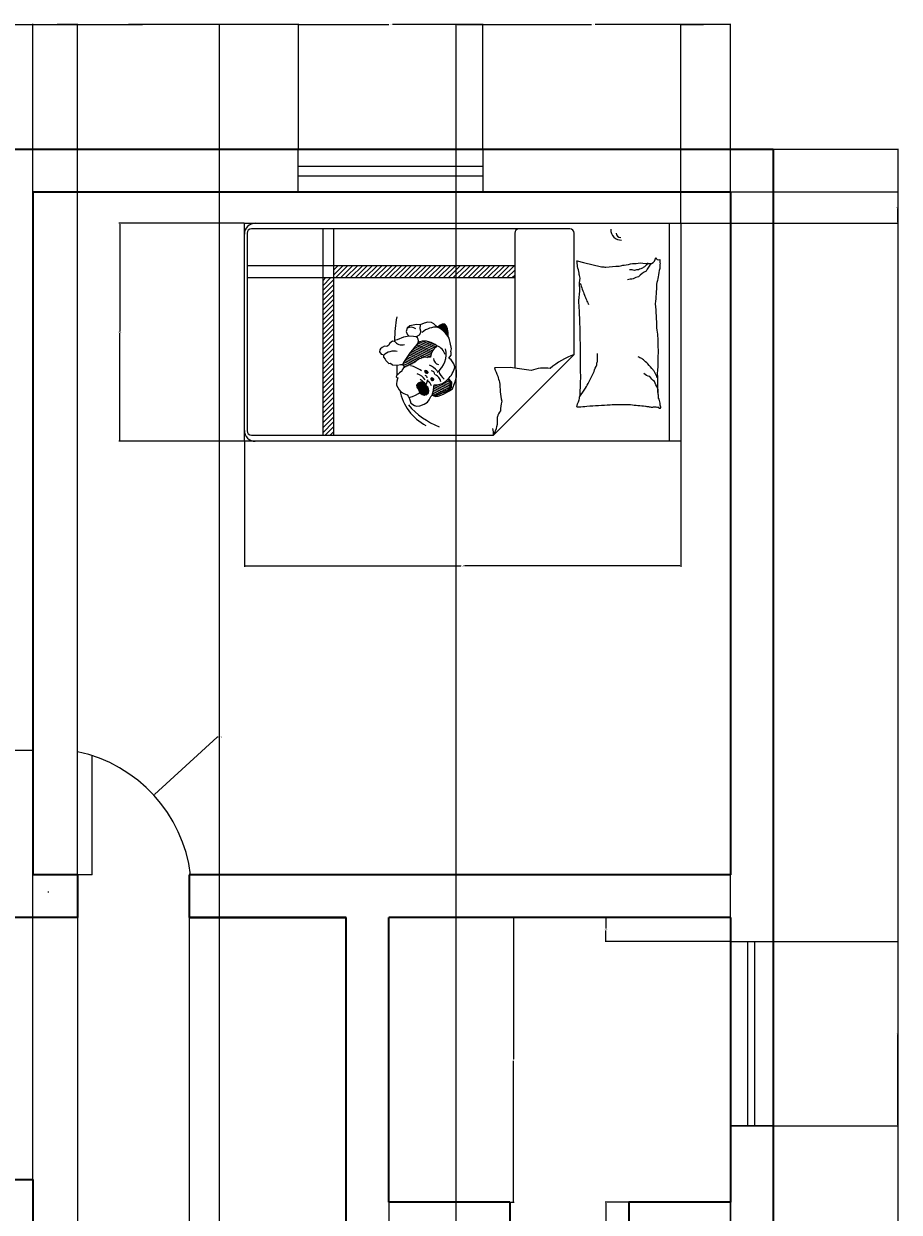
# Model space of a CAD drawing. Units: inches. Extents: x -20 to 351, y -512 to 63.
# Tile 5 of 5: x 166 to 351, y -188 to 63. Entities that reach past the tile are written whole.
import ezdxf

# ---------------------------------------------------------------- set-up
doc = ezdxf.new("R2010")
doc.units = ezdxf.units.IN
doc.header["$MEASUREMENT"] = 0
for name, color, linetype, lineweight in [('A-ANNO-DIMS', 2, 'Continuous', 18), ('A-DOOR', 3, 'Continuous', 18), ('A-FURN', 30, 'Continuous', 18), ('A-FURN-PATT', 30, 'Continuous', 9), ('A-GLAZ', 4, 'Continuous', 18), ('A-WALL', 7, 'Continuous', 35)]:
    doc.layers.add(name, color=color, linetype=linetype, lineweight=lineweight)
doc.styles.get("Standard").update_dxf_attribs({"font": 'arial.ttf'})
doc.dimstyles.get("Standard").update_dxf_attribs({"dimtxt": 0.18, "dimasz": 0.18, "dimexe": 0.18, "dimexo": 0.0625, "dimgap": 0.09, "dimtad": 0, "dimtih": 1, "dimtoh": 1, "dimdec": 4, "dimzin": 0, "dimdsep": 46, "dimtxsty": 'Standard', "dimcen": 0.09, "dimadec": 0, "dimazin": 0, "dimtfac": 1, "dimtdec": 4, "dimtofl": 0, "dimtmove": 0, "dimatfit": 3, "dimfxl": 1, "dimtolj": 1, "dimtzin": 0, "dimarcsym": 0})

# ---------------------------------------------------------------- blocks, each defined once
blk = doc.blocks.new('*D10')
at = {"layer": 'A-ANNO-DIMS', "color": 0, "lineweight": -2, "transparency": 16777216}
for p, q in [((324.35, 36.24), (350.71, 36.24)), ((350.53, 36.06), (350.53, -224.58)), ((350.53, -485.58), (350.53, -224.95)), ((324.35, -485.76), (350.71, -485.76))]:
    blk.add_line(p, q, dxfattribs=at)
at = {"layer": 'A-ANNO-DIMS', "color": 0, "transparency": 16777216}
for points in [[(350.5, 36.06), (350.56, 36.06), (350.53, 36.24)], [(350.5, -485.58), (350.56, -485.58), (350.53, -485.76)]]:
    blk.add_solid(points, dxfattribs=at)
at = {"layer": 'Defpoints', "color": 0, "transparency": 16777216}
for p in [(324.28, 36.24), (324.28, -485.76), (350.53, -485.76)]:
    blk.add_point(p, dxfattribs=at)
at = {"layer": 'A-ANNO-DIMS', "color": 0, "transparency": 16777216, "insert": (350.53, -224.76), "char_height": 0.18, "attachment_point": 5}
blk.add_mtext('\\A1;522', dxfattribs=at)
blk = doc.blocks.new('*D13')
at = {"layer": 'A-ANNO-DIMS', "color": 0, "lineweight": -2, "transparency": 16777216}
for p, q in [((159.28, 27.3), (159.28, 62.67)), ((224.21, 36.3), (224.21, 62.67)), ((159.46, 62.49), (191.35, 62.49)), ((224.03, 62.49), (192.14, 62.49))]:
    blk.add_line(p, q, dxfattribs=at)
at = {"layer": 'A-ANNO-DIMS', "color": 0, "transparency": 16777216}
for points in [[(159.46, 62.52), (159.46, 62.46), (159.28, 62.49)], [(224.03, 62.52), (224.03, 62.46), (224.21, 62.49)]]:
    blk.add_solid(points, dxfattribs=at)
at = {"layer": 'Defpoints', "color": 0, "transparency": 16777216}
for p in [(224.21, 62.49), (224.21, 36.24), (159.28, 27.24)]:
    blk.add_point(p, dxfattribs=at)
at = {"layer": 'A-ANNO-DIMS', "color": 0, "transparency": 16777216, "insert": (191.74, 62.49), "char_height": 0.18, "attachment_point": 5}
blk.add_mtext('\\A1;64.92', dxfattribs=at)
blk = doc.blocks.new('*D14')
at = {"layer": 'A-ANNO-DIMS', "color": 0, "lineweight": -2, "transparency": 16777216}
for p, q in [((224.21, 36.3), (224.21, 62.67)), ((263.09, 36.3), (263.09, 62.67)), ((224.39, 62.49), (243.25, 62.49)), ((262.91, 62.49), (244.04, 62.49))]:
    blk.add_line(p, q, dxfattribs=at)
at = {"layer": 'A-ANNO-DIMS', "color": 0, "transparency": 16777216}
for points in [[(224.39, 62.52), (224.39, 62.46), (224.21, 62.49)], [(262.91, 62.52), (262.91, 62.46), (263.09, 62.49)]]:
    blk.add_solid(points, dxfattribs=at)
at = {"layer": 'Defpoints', "color": 0, "transparency": 16777216}
for p in [(263.09, 62.49), (224.21, 36.24), (263.09, 36.24)]:
    blk.add_point(p, dxfattribs=at)
at = {"layer": 'A-ANNO-DIMS', "color": 0, "transparency": 16777216, "insert": (243.65, 62.49), "char_height": 0.18, "attachment_point": 5}
blk.add_mtext('\\A1;38.88', dxfattribs=at)
blk = doc.blocks.new('*D23')
at = {"layer": 'A-ANNO-DIMS', "color": 0, "lineweight": -2, "transparency": 16777216}
for p, q in [((315.22, -125.76), (288.85, -125.76)), ((289.03, -125.94), (289.03, -128.08)), ((289.03, -130.59), (289.03, -128.45)), ((315.22, -130.77), (288.85, -130.77))]:
    blk.add_line(p, q, dxfattribs=at)
at = {"layer": 'A-ANNO-DIMS', "color": 0, "transparency": 16777216}
for points in [[(289, -125.94), (289.06, -125.94), (289.03, -125.76)], [(289, -130.59), (289.06, -130.59), (289.03, -130.77)]]:
    blk.add_solid(points, dxfattribs=at)
at = {"layer": 'Defpoints', "color": 0, "transparency": 16777216}
for p in [(289.03, -125.76), (315.28, -125.76), (315.28, -130.77)]:
    blk.add_point(p, dxfattribs=at)
at = {"layer": 'A-ANNO-DIMS', "color": 0, "transparency": 16777216, "insert": (289.03, -128.26), "char_height": 0.18, "attachment_point": 5}
blk.add_mtext('\\A1;5.001', dxfattribs=at)
blk = doc.blocks.new('*D24')
at = {"layer": 'A-ANNO-DIMS', "color": 0, "lineweight": -2, "transparency": 16777216}
for p, q in [((324.35, -130.77), (350.71, -130.77)), ((350.53, -130.95), (350.53, -150.02)), ((350.53, -169.47), (350.53, -150.39)), ((324.35, -169.65), (350.71, -169.65))]:
    blk.add_line(p, q, dxfattribs=at)
at = {"layer": 'A-ANNO-DIMS', "color": 0, "transparency": 16777216}
for points in [[(350.5, -130.95), (350.56, -130.95), (350.53, -130.77)], [(350.5, -169.47), (350.56, -169.47), (350.53, -169.65)]]:
    blk.add_solid(points, dxfattribs=at)
at = {"layer": 'Defpoints', "color": 0, "transparency": 16777216}
for p in [(324.28, -130.77), (324.28, -169.65), (350.53, -169.65)]:
    blk.add_point(p, dxfattribs=at)
at = {"layer": 'A-ANNO-DIMS', "color": 0, "transparency": 16777216, "insert": (350.53, -150.21), "char_height": 0.18, "attachment_point": 5}
blk.add_mtext('\\A1;38.88', dxfattribs=at)
blk = doc.blocks.new('*D25')
at = {"layer": 'A-ANNO-DIMS', "color": 0, "lineweight": -2, "transparency": 16777216}
for p, q in [((315.22, -185.76), (288.85, -185.76)), ((289.03, -185.94), (289.03, -231.17)), ((289.03, -276.76), (289.03, -231.53)), ((315.22, -276.94), (288.85, -276.94))]:
    blk.add_line(p, q, dxfattribs=at)
at = {"layer": 'A-ANNO-DIMS', "color": 0, "transparency": 16777216}
for points in [[(289, -185.94), (289.06, -185.94), (289.03, -185.76)], [(289, -276.76), (289.06, -276.76), (289.03, -276.94)]]:
    blk.add_solid(points, dxfattribs=at)
at = {"layer": 'Defpoints', "color": 0, "transparency": 16777216}
for p in [(289.03, -185.76), (315.28, -185.76), (315.28, -276.94)]:
    blk.add_point(p, dxfattribs=at)
at = {"layer": 'A-ANNO-DIMS', "color": 0, "transparency": 16777216, "insert": (289.03, -231.35), "char_height": 0.18, "attachment_point": 5}
blk.add_mtext('\\A1;91.18', dxfattribs=at)
blk = doc.blocks.new('*D33')
at = {"layer": 'A-ANNO-DIMS', "color": 0, "lineweight": -2, "transparency": 16777216}
for p, q in [((159.28, -116.7), (159.28, -90.33)), ((159.46, -90.51), (163.64, -90.51)), ((168.1, -90.51), (163.93, -90.51)), ((168.28, -116.7), (168.28, -90.33))]:
    blk.add_line(p, q, dxfattribs=at)
at = {"layer": 'A-ANNO-DIMS', "color": 0, "transparency": 16777216}
for points in [[(159.46, -90.48), (159.46, -90.54), (159.28, -90.51)], [(168.1, -90.48), (168.1, -90.54), (168.28, -90.51)]]:
    blk.add_solid(points, dxfattribs=at)
at = {"layer": 'Defpoints', "color": 0, "transparency": 16777216}
for p in [(168.28, -90.51), (159.28, -116.76), (168.28, -116.76)]:
    blk.add_point(p, dxfattribs=at)
at = {"layer": 'A-ANNO-DIMS', "color": 0, "transparency": 16777216, "insert": (163.78, -90.51), "char_height": 0.18, "attachment_point": 5}
blk.add_mtext('\\A1;9', dxfattribs=at)
blk = doc.blocks.new('*D37')
at = {"layer": 'A-ANNO-DIMS', "color": 0, "lineweight": -2, "transparency": 16777216}
for p, q in [((243.28, -125.83), (243.28, -512.19)), ((315.28, -125.83), (315.28, -512.19)), ((243.46, -512.01), (279.07, -512.01)), ((315.1, -512.01), (279.5, -512.01))]:
    blk.add_line(p, q, dxfattribs=at)
at = {"layer": 'A-ANNO-DIMS', "color": 0, "transparency": 16777216}
for points in [[(243.46, -511.98), (243.46, -512.04), (243.28, -512.01)], [(315.1, -511.98), (315.1, -512.04), (315.28, -512.01)]]:
    blk.add_solid(points, dxfattribs=at)
at = {"layer": 'Defpoints', "color": 0, "transparency": 16777216}
for p in [(243.28, -125.76), (315.28, -125.76), (315.28, -512.01)]:
    blk.add_point(p, dxfattribs=at)
at = {"layer": 'A-ANNO-DIMS', "color": 0, "transparency": 16777216, "insert": (279.28, -512.01), "char_height": 0.18, "attachment_point": 5}
blk.add_mtext('\\A1;72', dxfattribs=at)
blk = doc.blocks.new('*D38')
at = {"layer": 'A-ANNO-DIMS', "color": 0, "lineweight": -2, "transparency": 16777216}
for p, q in [((243.35, -125.76), (269.71, -125.76)), ((269.53, -125.94), (269.53, -155.58)), ((269.53, -185.58), (269.53, -155.95)), ((243.35, -185.76), (269.71, -185.76))]:
    blk.add_line(p, q, dxfattribs=at)
at = {"layer": 'A-ANNO-DIMS', "color": 0, "transparency": 16777216}
for points in [[(269.5, -125.94), (269.56, -125.94), (269.53, -125.76)], [(269.5, -185.58), (269.56, -185.58), (269.53, -185.76)]]:
    blk.add_solid(points, dxfattribs=at)
at = {"layer": 'Defpoints', "color": 0, "transparency": 16777216}
for p in [(243.28, -125.76), (243.28, -185.76), (269.53, -185.76)]:
    blk.add_point(p, dxfattribs=at)
at = {"layer": 'A-ANNO-DIMS', "color": 0, "transparency": 16777216, "insert": (269.53, -155.76), "char_height": 0.18, "attachment_point": 5}
blk.add_mtext('\\A1;60', dxfattribs=at)
blk = doc.blocks.new('*D41')
at = {"layer": 'A-ANNO-DIMS', "color": 0, "lineweight": -2, "transparency": 16777216}
for p, q in [((168.28, -116.7), (168.28, 62.67)), ((177.69, -116.7), (177.69, 62.67)), ((168.46, 62.49), (172.59, 62.49)), ((177.51, 62.49), (173.38, 62.49))]:
    blk.add_line(p, q, dxfattribs=at)
at = {"layer": 'A-ANNO-DIMS', "color": 0, "transparency": 16777216}
for points in [[(168.46, 62.52), (168.46, 62.46), (168.28, 62.49)], [(177.51, 62.52), (177.51, 62.46), (177.69, 62.49)]]:
    blk.add_solid(points, dxfattribs=at)
at = {"layer": 'Defpoints', "color": 0, "transparency": 16777216}
for p in [(177.69, 62.49), (168.28, -116.76), (177.69, -116.76)]:
    blk.add_point(p, dxfattribs=at)
at = {"layer": 'A-ANNO-DIMS', "color": 0, "transparency": 16777216, "insert": (172.99, 62.49), "char_height": 0.18, "attachment_point": 5}
blk.add_mtext('\\A1;9.404', dxfattribs=at)
blk = doc.blocks.new('*D42')
at = {"layer": 'A-ANNO-DIMS', "color": 0, "lineweight": -2, "transparency": 16777216}
for p, q in [((177.69, -125.83), (177.69, -512.19)), ((201.2, -125.83), (201.2, -512.19)), ((177.87, -512.01), (188.98, -512.01)), ((201.02, -512.01), (189.91, -512.01))]:
    blk.add_line(p, q, dxfattribs=at)
at = {"layer": 'A-ANNO-DIMS', "color": 0, "transparency": 16777216}
for points in [[(177.87, -511.98), (177.87, -512.04), (177.69, -512.01)], [(201.02, -511.98), (201.02, -512.04), (201.2, -512.01)]]:
    blk.add_solid(points, dxfattribs=at)
at = {"layer": 'Defpoints', "color": 0, "transparency": 16777216}
for p in [(177.69, -125.76), (201.2, -125.76), (201.2, -512.01)]:
    blk.add_point(p, dxfattribs=at)
at = {"layer": 'A-ANNO-DIMS', "color": 0, "transparency": 16777216, "insert": (189.45, -512.01), "char_height": 0.18, "attachment_point": 5}
blk.add_mtext('\\A1;23.516', dxfattribs=at)
blk = doc.blocks.new('*D57')
at = {"layer": 'A-ANNO-DIMS', "color": 0, "lineweight": -2, "transparency": 16777216}
for p, q in [((212.84, -25.42), (212.84, -51.78)), ((304.8, -25.42), (304.8, -51.78)), ((213.02, -51.6), (258.42, -51.6)), ((304.62, -51.6), (259.21, -51.6))]:
    blk.add_line(p, q, dxfattribs=at)
at = {"layer": 'A-ANNO-DIMS', "color": 0, "transparency": 16777216}
for points in [[(213.02, -51.57), (213.02, -51.63), (212.84, -51.6)], [(304.62, -51.57), (304.62, -51.63), (304.8, -51.6)]]:
    blk.add_solid(points, dxfattribs=at)
at = {"layer": 'Defpoints', "color": 0, "transparency": 16777216}
for p in [(212.84, -25.35), (304.8, -25.35), (212.84, -51.6)]:
    blk.add_point(p, dxfattribs=at)
at = {"layer": 'A-ANNO-DIMS', "color": 0, "transparency": 16777216, "insert": (258.82, -51.6), "char_height": 0.18, "attachment_point": 5}
blk.add_mtext('\\A1;91.96', dxfattribs=at)
blk = doc.blocks.new('*D58')
at = {"layer": 'A-ANNO-DIMS', "color": 0, "lineweight": -2, "transparency": 16777216}
for p, q in [((212.78, 20.63), (186.41, 20.63)), ((186.59, 20.45), (186.59, -2.18)), ((186.59, -25.17), (186.59, -2.55)), ((212.78, -25.35), (186.41, -25.35))]:
    blk.add_line(p, q, dxfattribs=at)
at = {"layer": 'A-ANNO-DIMS', "color": 0, "transparency": 16777216}
for points in [[(186.56, 20.45), (186.62, 20.45), (186.59, 20.63)], [(186.56, -25.17), (186.62, -25.17), (186.59, -25.35)]]:
    blk.add_solid(points, dxfattribs=at)
at = {"layer": 'Defpoints', "color": 0, "transparency": 16777216}
for p in [(186.59, 20.63), (212.84, 20.63), (212.84, -25.35)]:
    blk.add_point(p, dxfattribs=at)
at = {"layer": 'A-ANNO-DIMS', "color": 0, "transparency": 16777216, "insert": (186.59, -2.36), "char_height": 0.18, "attachment_point": 5}
blk.add_mtext('\\A1;45.98', dxfattribs=at)
blk = doc.blocks.new('*D59')
at = {"layer": 'A-ANNO-DIMS', "color": 0, "lineweight": -2, "transparency": 16777216}
for p, q in [((304.8, 20.69), (304.8, 62.67)), ((315.28, 27.3), (315.28, 62.67)), ((304.98, 62.49), (309.59, 62.49)), ((315.1, 62.49), (310.5, 62.49))]:
    blk.add_line(p, q, dxfattribs=at)
at = {"layer": 'A-ANNO-DIMS', "color": 0, "transparency": 16777216}
for points in [[(304.98, 62.52), (304.98, 62.46), (304.8, 62.49)], [(315.1, 62.52), (315.1, 62.46), (315.28, 62.49)]]:
    blk.add_solid(points, dxfattribs=at)
at = {"layer": 'Defpoints', "color": 0, "transparency": 16777216}
for p in [(315.28, 62.49), (315.28, 27.24), (304.8, 20.63)]:
    blk.add_point(p, dxfattribs=at)
at = {"layer": 'A-ANNO-DIMS', "color": 0, "transparency": 16777216, "insert": (310.04, 62.49), "char_height": 0.18, "attachment_point": 5}
blk.add_mtext('\\A1;10.488', dxfattribs=at)
blk = doc.blocks.new('*D60')
at = {"layer": 'A-ANNO-DIMS', "color": 0, "lineweight": -2, "transparency": 16777216}
for p, q in [((315.35, 27.24), (350.71, 27.24)), ((350.53, 27.06), (350.53, 24.11)), ((350.53, 20.81), (350.53, 23.75)), ((304.86, 20.63), (350.71, 20.63))]:
    blk.add_line(p, q, dxfattribs=at)
at = {"layer": 'A-ANNO-DIMS', "color": 0, "transparency": 16777216}
for points in [[(350.5, 27.06), (350.56, 27.06), (350.53, 27.24)], [(350.5, 20.81), (350.56, 20.81), (350.53, 20.63)]]:
    blk.add_solid(points, dxfattribs=at)
at = {"layer": 'Defpoints', "color": 0, "transparency": 16777216}
for p in [(315.28, 27.24), (350.53, 27.24), (304.8, 20.63)]:
    blk.add_point(p, dxfattribs=at)
at = {"layer": 'A-ANNO-DIMS', "color": 0, "transparency": 16777216, "insert": (350.53, 23.93), "char_height": 0.18, "attachment_point": 5}
blk.add_mtext('\\A1;6.61', dxfattribs=at)
blk = doc.blocks.new('*D61')
at = {"layer": 'A-ANNO-DIMS', "color": 0, "lineweight": -2, "transparency": 16777216}
for p, q in [((168.28, -269.91), (168.28, 62.67)), ((207.59, -267.77), (207.59, 62.67)), ((168.46, 62.49), (187.47, 62.49)), ((207.41, 62.49), (188.4, 62.49))]:
    blk.add_line(p, q, dxfattribs=at)
at = {"layer": 'A-ANNO-DIMS', "color": 0, "transparency": 16777216}
for points in [[(168.46, 62.52), (168.46, 62.46), (168.28, 62.49)], [(207.41, 62.52), (207.41, 62.46), (207.59, 62.49)]]:
    blk.add_solid(points, dxfattribs=at)
at = {"layer": 'Defpoints', "color": 0, "transparency": 16777216}
for p in [(207.59, 62.49), (207.59, -267.83), (168.28, -269.98)]:
    blk.add_point(p, dxfattribs=at)
at = {"layer": 'A-ANNO-DIMS', "color": 0, "transparency": 16777216, "insert": (187.94, 62.49), "char_height": 0.18, "attachment_point": 5}
blk.add_mtext('\\A1;39.305', dxfattribs=at)
blk = doc.blocks.new('*D62')
at = {"layer": 'A-ANNO-DIMS', "color": 0, "lineweight": -2, "transparency": 16777216}
for p, q in [((257.5, -263.86), (257.5, 62.67)), ((315.28, -276.88), (315.28, 62.67)), ((257.68, 62.49), (286, 62.49)), ((315.1, 62.49), (286.79, 62.49))]:
    blk.add_line(p, q, dxfattribs=at)
at = {"layer": 'A-ANNO-DIMS', "color": 0, "transparency": 16777216}
for points in [[(257.68, 62.52), (257.68, 62.46), (257.5, 62.49)], [(315.1, 62.52), (315.1, 62.46), (315.28, 62.49)]]:
    blk.add_solid(points, dxfattribs=at)
at = {"layer": 'Defpoints', "color": 0, "transparency": 16777216}
for p in [(315.28, 62.49), (257.5, -263.93), (315.28, -276.94)]:
    blk.add_point(p, dxfattribs=at)
at = {"layer": 'A-ANNO-DIMS', "color": 0, "transparency": 16777216, "insert": (286.39, 62.49), "char_height": 0.18, "attachment_point": 5}
blk.add_mtext('\\A1;57.78', dxfattribs=at)
blk = doc.blocks.new('*D77')
at = {"layer": 'A-ANNO-DIMS', "color": 0, "lineweight": -2, "transparency": 16777216}
for p, q in [((207.1, -87.73), (193.9, -99.84)), ((207.28, -87.73), (207.1, -87.73)), ((171.44, -120.35), (171.62, -120.35)), ((171.53, -120.44), (171.53, -120.26))]:
    blk.add_line(p, q, dxfattribs=at)
at = {"layer": 'A-ANNO-DIMS', "color": 0, "transparency": 16777216}
blk.add_solid([(193.88, -99.82), (193.92, -99.86), (193.76, -99.96)], dxfattribs=at)
at = {"layer": 'Defpoints', "color": 0, "transparency": 16777216}
for p in [(193.76, -99.96), (171.53, -120.35)]:
    blk.add_point(p, dxfattribs=at)
at = {"layer": 'A-ANNO-DIMS', "color": 0, "transparency": 16777216, "insert": (207.76, -87.73), "char_height": 0.18, "attachment_point": 5}
blk.add_mtext('\\A1;R30.17', dxfattribs=at)

msp = doc.modelspace()

# ---------------------------------------------------------------- hatches: boundary and pattern name
at = {"layer": 'A-FURN-PATT'}
h = msp.add_hatch(dxfattribs=at)
h.set_pattern_fill('ANSI31', color=256, scale=0.229896, angle=-90, style=0)
h.set_pattern_definition([(45, (336.464, -36.1554), (0.5161305, -0.5161305), [])])
h.paths.add_polyline_path([(231.5979, 9.1557), (269.8006, 9.1557), (269.8006, 11.7278), (231.5979, 11.7278)])
h.paths.add_polyline_path([(231.5979, 9.1557), (229.345, 9.1557), (229.345, -24.0467), (231.5979, -24.0467)])
h = msp.add_hatch(dxfattribs=at)
h.set_pattern_fill('ANSI31', color=256, scale=1.379374, angle=-67.191735, style=0)
h.set_pattern_definition([(337.808265, (1189.52844, -405.23684), (0.065124935, 0.159649613), [])])
h.paths.add_polyline_path([(255.7673, -3.2568), (255.7568, -3.2318), (255.791, -2.4906), (255.6458, -1.6518), (255.4278, -1.0513), (255.0536, -0.6549), (254.4967, -0.6468), (254.0976, -0.8492), (253.7356, -1.1399), (253.5546, -1.2852, -0.12950097)])
h = msp.add_hatch(dxfattribs=at)
h.set_pattern_fill('ANSI31', color=256, scale=2.758748, angle=-67.191735, style=0)
h.set_pattern_definition([(337.808265, (1189.52844, -405.23684), (0.13024987, 0.31929923), [])])
h.paths.add_polyline_path([(254.5946, -13.1347), (253.8645, -13.3725), (252.8297, -13.4616), (252.7646, -13.8004), (252.6794, -14.6669), (252.4996, -15.301), (253.2268, -15.475), (254.0667, -15.0872), (255.7203, -14.4956), (256.1427, -13.9373), (256.2125, -12.8696), (255.6806, -12.2627), (255.2799, -12.7081)])
h.paths.add_polyline_path([(252.039, -7.6342, -0.19504951), (253.4239, -5.2521, 0.24235496), (249.7954, -4.3552, 0.07086884), (246.1683, -9.1822), (246.4162, -9.4787), (246.7333, -9.6569), (247.6738, -9.2623), (248.7829, -8.692), (249.5533, -8.0566), (250.5479, -7.7075)])
h = msp.add_hatch(dxfattribs=at)
h.set_pattern_fill('ANSI31', color=256, scale=0.651754, angle=-67.191735, style=0)
h.set_pattern_definition([(337.808265, (1141.0097, -409.06169), (0.030771532, 0.075434442), [])])
h.paths.add_polyline_path([(251.2068, -10.9907), (251.4546, -10.9678), (251.5897, -10.8704), (251.4583, -10.6545), (251.2821, -10.5253), (250.9398, -10.4524), (250.8047, -10.5499), (250.8707, -10.739), (250.9991, -10.9154)])
h.paths.add_polyline_path([(252.3216, -12.5143), (252.5167, -12.5272), (252.7172, -12.4564), (252.7802, -12.3486), (252.7742, -12.2698), (252.6585, -12.1558), (252.5216, -12.0236), (252.2775, -11.9907), (252.1261, -12.0815), (252.1133, -12.2766)])
h = msp.add_hatch(dxfattribs=at)
h.set_pattern_fill('ANSI31', color=256, scale=1.629385, angle=-67.191735, style=0)
h.set_pattern_definition([(337.808265, (1141.0097, -409.0617), (0.07692883, 0.188586106), [])])
h.paths.add_polyline_path([(251.26, -13.768), (250.9538, -13.1878), (250.806, -13.0136), (250.5675, -12.89), (250.3813, -12.8314), (249.9672, -12.8812), (249.4946, -13.1173), (249.1126, -13.5391), (249.1898, -13.9296), (249.5521, -14.4365), (249.661, -14.8136), (249.8322, -15.1024), (250.3352, -15.5004), (250.7465, -15.6508), (251.2485, -15.5143), (251.6121, -15.1375), (251.7112, -14.7227), (251.6712, -14.3912), (251.5073, -13.9128)])

# ---------------------------------------------------------------- linework, layer by layer
at = {"layer": 'A-DOOR'}
for p, q in [((177.6888, -116.7646), (177.6888, -90.8152)), ((180.7602, -116.7646), (180.7602, -91.6268)), ((177.6888, -116.7646), (177.6888, -116.7646)), ((180.7602, -116.7646), (177.6888, -116.7646))]:
    msp.add_line(p, q, dxfattribs=at)
msp.add_arc((171.5283, -120.3465), 30.1671, 6.819192, 78.216438, dxfattribs=at)
at = {"layer": 'A-FURN'}
for p, q in [((212.8384, 20.6254), (304.7967, 20.6254)), ((212.8384, -25.3538), (212.8384, 20.6254)), ((302.3887, 20.6254), (302.3887, -25.3538)), ((304.7967, 20.6254), (304.7967, -25.3538)), ((213.398, 18.5187), (213.398, -23.1271)), ((281.4149, 19.4383), (214.3176, 19.4383)), ((229.345, 19.4383), (229.345, -24.0467)), ((231.5979, 19.4383), (231.5979, -24.0467)), ((269.8006, 18.5187), (269.8006, -9.9248)), ((282.3345, -7.0833), (282.3345, 18.5187)), ((282.3345, -7.0833), (265.3322, -24.0467)), ((214.3176, -24.0467), (265.3322, -24.0467)), ((304.7967, -25.3538), (212.8384, -25.3538))]:
    msp.add_line(p, q, dxfattribs=at)
for points in [[(298.6535, 12.1156, 0.26336794), (299.5174, 13.4007, 0.49481805), (300.3792, 12.979, 0.04922472), (300.4594, 12.1665, 0.03683084), (300.3792, 11.0795, 0.03189269), (300.0052, 9.3333, -0.035782), (299.6838, 7.7739, -0.03294126), (299.4119, 3.6514, -0.02656446), (299.6838, -1.4628, -0.01790542), (299.9304, -3.1876, 0.00966744), (300.0341, -6.4157, 0.03203963), (300.0004, -8.1208, -0.01844195), (299.8615, -11.0782, -0.01083729), (299.8961, -14.056, -0.01462385), (300.0341, -16.2588, -0.11124937), (300.37, -17.2955, 0.15370834), (300.5518, -18.072, 0.07644442), (300.4726, -18.4139, 0.21551229), (300.3792, -18.5037, 0.58585823), (300.2392, -18.3813, -0.36348931), (300.1204, -18.1583, -0.19171627), (299.59, -18.1557, 0.1296753), (298.8261, -18.2446, 0.01735021), (298.0535, -18.1067, -0.01932565), (297.3593, -17.9856, -0.01881752), (294.2151, -17.6815, -0.0218281), (291.492, -17.6403, -0.00620415), (289.9355, -17.704, -0.00196306), (285.0206, -17.9856, -0.02834083), (283.3595, -18.1823, 0.11701353), (282.9498, -18.1583, 0.36605999), (282.907, -18.0926, 0.03973043), (283.0361, -17.4676, 0.04830882), (283.2881, -16.8359, -0.06298072), (283.4675, -16.3451, -0.04057963), (283.623, -15.2693, -0.01434509), (283.7264, -12.2007, -0.00548442), (283.692, -6.4328, -0.00470685), (283.5538, 0.2867, -0.00876157), (283.4303, 2.2428, 0.00815313), (283.295, 4.3448, 0.06251003), (283.4973, 6.9715, -0.07866929), (283.5911, 9.0676, -0.04782509), (283.3742, 10.0957, 0.03449399), (283.0361, 11.5112, 0.02357139), (282.8975, 12.6761, 0.51022848), (282.9498, 12.72), (284.3304, 12.3746), (288.1269, 11.4248, -0.07304094), (289.0272, 11.3351, -0.0233051), (291.8371, 11.5975, -0.01829889), (292.8875, 11.7847, 0.01096989), (294.6344, 12.1224, 0.04228119), (296.2121, 12.256, 0.02720053), (298.6671, 12.1224)], [(298.6542, 12.1238, 0.07737943), (297.489, 10.5232, 0.07737943), (295.8924, 9.3526, 0.04752549), (294.7605, 8.8963, 0.04752549), (293.5628, 8.6619)], [(297.9171, 12.1917, 0.05368995), (297.3204, 11.5385, 0.07031175), (296.7553, 11.1658, 0.01544823), (296.362, 10.9941, 0.01324357), (295.8924, 10.8204, 0.08212667), (295.0611, 10.683, 0.0641637), (293.9942, 10.8204)], [(283.6239, 7.9595, -0.00972947), (284.0392, 6.7048, -0.00972947), (284.5029, 5.4672, -0.0079705), (284.9185, 4.4674, -0.0079705), (285.3658, 3.4813)], [(282.3345, -7.0833, 0.08527182), (277.2719, -9.9941, 0.12404448), (273.2474, -10.4175), (268.8605, -9.7904), (265.5258, -9.8707)], [(283.5538, -15.9134, -0.01610775), (284.7599, -14.124, -0.02459883), (285.4521, -12.8914, -0.00947722), (286.5233, -10.6367, -0.01593728), (287.0915, -9.265, -0.07252085), (287.2564, -8.5137, -0.03333928), (287.264, -6.8475)], [(299.8583, -11.9711, -0.02784216), (299.3704, -10.8776, -0.04868501), (298.9987, -10.3012, -0.02366646), (297.8787, -9.0173, -0.03122342), (296.9279, -8.1426, -0.04680097), (296.5754, -7.9077, -0.02319083), (295.8062, -7.5382)], [(300.1204, -15.7407, -0.08815313), (299.9574, -14.1531, -0.08815313), (299.2575, -12.7187, -0.07754712), (298.2638, -11.7235, -0.07754712), (297.0141, -11.0782)]]:
    msp.add_lwpolyline(points, format="xyb", dxfattribs=at)
for points in [[(213.398, 11.7278), (269.8006, 11.7278)], [(213.398, 9.1557), (269.8006, 9.1557)], [(253.5546, -1.2852), (253.267, -1.0947), (252.7721, -0.576), (252.3051, -0.2878), (251.5225, -0.2362), (250.6918, -0.4817), (249.8982, -0.8154), (249.1326, -0.7221), (248.0344, -0.907), (247.6864, -0.9841), (247.1093, -1.5037), (246.9081, -2.1767), (247.1137, -2.7478), (247.5544, -3.2201), (246.3974, -3.4298), (245.0625, -3.9566), (244.4793, -4.1326), (244.4236, -4.3291), (244.0849, -4.2638), (243.4119, -4.7199), (243.3005, -5.1129), (242.8426, -5.34), (242.3739, -5.2948), (241.8403, -5.5885), (241.5247, -5.825), (241.3637, -6.1004), (241.2941, -6.5104), (241.6636, -6.978), (242.0859, -7.0773), (242.1601, -7.2537), (242.1786, -7.6267), (242.5234, -8.0354), (242.6177, -8.3419), (243.2796, -8.9288), (243.6523, -8.9105), (244.0188, -9.2063), (245.1402, -9.3231), (245.7357, -9.1765), (246.1379, -9.1459), (246.4162, -9.4787), (246.7333, -9.6569), (246.3249, -10.0017), (246.0634, -10.2847), (246.0448, -10.5694), (245.5235, -10.8925), (245.262, -11.1755), (244.9758, -11.3997), (244.8396, -11.7338), (244.9556, -11.9274), (245.169, -11.9414), (245.1381, -12.1967), (244.9802, -12.6438), (244.8965, -13.2674), (244.9243, -13.498), (245.2057, -14.0026), (245.4577, -14.5197), (245.8026, -14.9284), (246.4073, -15.2971), (247.1636, -15.5328), (247.3584, -15.8316), (247.6522, -16.3657), (247.7665, -16.8021), (247.9474, -17.3145), (248.6851, -17.8349), (249.1367, -17.9219), (249.8111, -17.8805), (250.6928, -17.5097), (251.4322, -17.1296), (251.7788, -16.6377), (252.1564, -15.8906), (252.4008, -15.6493), (253.1107, -15.9392), (253.7016, -15.8637), (254.772, -15.4482), (255.264, -15.1375), (256.0622, -14.7326), (256.7057, -14.2889), (257.0121, -13.5371), (257.2597, -12.81), (257.543, -11.7563), (257.5433, -10.441), (257.4707, -10.0216), (257.1676, -9.6299), (256.9497, -9.0293), (256.4317, -8.2089), (255.9569, -7.8201), (256.3963, -7.22), (256.4506, -6.6088), (256.347, -6.4447), (256.4848, -5.8676), (256.1881, -4.5041), (256.066, -3.9671), (255.9887, -3.6188), (255.831, -3.4083), (255.7568, -3.2318), (255.791, -2.4906), (255.6458, -1.6518), (255.4278, -1.0513), (255.0536, -0.6549), (254.4967, -0.6468), (254.0976, -0.8492), (253.7356, -1.1399), (253.5546, -1.2852)], [(249.8982, -0.8154), (249.847, -1.5993), (249.9969, -2.3669), (249.641, -3.0011), (249.0191, -3.3319), (248.467, -3.2526), (247.5544, -3.2201)], [(252.039, -7.6342), (250.5479, -7.7075), (249.5533, -8.0566), (248.7829, -8.692), (247.6738, -9.2623), (246.7333, -9.6569)], [(251.2821, -10.5253), (250.9398, -10.4524), (250.8047, -10.5499), (250.8707, -10.739), (250.9991, -10.9154), (251.2068, -10.9907), (251.4546, -10.9678), (251.5897, -10.8704), (251.4583, -10.6545), (251.2821, -10.5253)], [(252.5216, -12.0236), (252.2775, -11.9907), (252.1261, -12.0815), (252.1133, -12.2766), (252.3216, -12.5143), (252.5167, -12.5272), (252.7172, -12.4564), (252.7802, -12.3486), (252.7742, -12.2698), (252.6585, -12.1558), (252.5216, -12.0236)], [(252.4008, -15.6493), (252.6794, -14.6669), (252.7646, -13.8004), (252.8297, -13.4616), (253.8645, -13.3725), (254.5946, -13.1347), (255.2799, -12.7081), (255.6806, -12.2627)], [(255.8712, -12.0956), (256.4723, -12.7815), (256.3907, -14.0296), (255.8769, -14.7088), (254.1627, -15.322), (253.2532, -15.742), (252.4406, -15.5475)], [(255.6806, -12.2627), (256.2125, -12.8696), (256.1427, -13.9373), (255.7203, -14.4956), (254.0667, -15.0872), (253.2268, -15.475), (252.4996, -15.301)], [(251.26, -13.768), (250.9538, -13.1878), (250.806, -13.0136), (250.5675, -12.89), (250.3813, -12.8314), (249.9672, -12.8812), (249.4946, -13.1173), (249.1126, -13.5391), (249.1898, -13.9296), (249.5521, -14.4365), (249.661, -14.8136), (249.8322, -15.1024), (250.3352, -15.5004), (250.7465, -15.6508), (251.2485, -15.5143), (251.6121, -15.1375), (251.7112, -14.7227), (251.6712, -14.3912), (251.5073, -13.9128), (251.26, -13.768)]]:
    msp.add_lwpolyline(points, dxfattribs=at)
for centre, radius, start, end in [((215.1374, 18.3264), 2.299, 90, 180), ((214.3176, 18.5187), 0.9196, 90, 180), ((270.7202, 18.5187), 0.9196, 90, 180), ((281.4149, 18.5187), 0.9196, 0, 90), ((292.3307, 19.3386), 2.299, 180, 270), ((292.1384, 18.5187), 0.9196, 180, 270), ((270.3511, -4.1117), 25.8718, 168.815296, 180.046298), ((247.9532, -3.1212), 1.8244, 54.832477, 117.551318), ((253.2913, -5.7546), 4.4771, 86.628328, 131.525417), ((250.9187, -6.4708), 5.8171, 29.358635, 63.055166), ((246.0726, -3.0167), 2.0254, 216.830277, 284.49505), ((264.9242, -19.4995), 21.4063, 134.970653, 151.185485), ((248.507, -4.2288), 1.0328, 343.07967, 60.275705), ((250.7388, -8.3268), 4.082, 48.869707, 103.362689), ((244.3495, -9.4503), 3.1013, 76.55539, 134.906173), ((255.6685, -8.1506), 3.666, 127.754681, 171.902449), ((252.5926, -7.7299), 2.6135, 14.732507, 71.455109), ((250.6555, -6.9942), 4.714, 306.614107, 13.933363), ((291.0243, -8.9347), 46.0937, 180.473367, 183.062835), ((247.0324, -14.2368), 4.8474, 50.113778, 80.242572), ((249.7158, -14.0668), 5.1984, 43.477802, 66.085659), ((254.1176, -7.7617), 1.4579, 185.5542, 255.95894), ((252.8989, -8.9552), 4.3217, 310.064606, 351.018441), ((282.093, -3.8578), 17.6245, 199.947792, 206.217173), ((246.8155, -11.3737), 4.775, 278.305372, 348.947321), ((248.37, -14.1824), 3.16, 34.800606, 74.271325), ((240.5067, -25.9368), 16.5182, 51.992749, 55.488636), ((250.8546, -11.9799), 0.504, 0.109736, 77.360097), ((252.1566, -11.3388), 0.8536, 4.247793, 86.558047), ((252.1254, -13.1928), 2.1193, 11.013967, 61.983793), ((257.1398, -9.5073), 3.5159, 197.628386, 231.982197), ((274.0744, -10.1863), 7.928, 190.594462, 199.947792), ((255.6268, -12.9245), 10.1338, 189.437122, 243.543195), ((250.1118, -13.7396), 0.6693, 184.953624, 347.058903), ((250.2691, -14.3332), 0.5996, 190.739531, 298.107344), ((250.4415, -14.0567), 0.8128, 277.778181, 5.183682), ((250.9814, -14.7517), 0.4438, 194.393793, 284.927002), ((250.5246, -14.1815), 1.8057, 16.623572, 57.032033), ((293.0068, -12.0671), 26.3976, 181.788715, 190.594462), ((273.5271, -18.7404), 6.7191, 164.283937, 181.788715), ((260.2902, -6.4744), 17.0804, 221.031377, 247.893398), ((269.4997, -21.1573), 3.4784, 140.613932, 164.283936), ((260.3354, -20.9751), 5.8653, 328.420081, 7.444324), ((215.1374, -23.0573), 2.299, 180, 270), ((214.3176, -23.1271), 0.9196, 180, 270), ((258.4713, -23.8785), 6.8629, 358.595696, 10.574456)]:
    msp.add_arc(centre, radius, start, end, dxfattribs=at)
at = {"layer": 'A-GLAZ'}
for p, q in [((263.0876, 32.5902), (224.2051, 32.5902)), ((263.0876, 30.5508), (224.2051, 30.5508)), ((318.871, -130.7652), (318.871, -169.6477)), ((320.3524, -130.7652), (320.3524, -169.6477)), ((315.2844, -169.6477), (324.2844, -169.6477))]:
    msp.add_line(p, q, dxfattribs=at)
for points in [[(263.0876, 36.2354), (263.0876, 27.2354), (224.2051, 27.2354), (224.2051, 36.2354)], [(315.2844, -130.7652), (324.2844, -130.7652), (324.2844, -169.6477), (315.2844, -169.6477)]]:
    msp.add_lwpolyline(points, close=True, dxfattribs=at)
at = {"layer": 'A-WALL'}
for p, q in [((6.2844, 36.2354), (324.2844, 36.2354)), ((324.2844, 36.2354), (324.2844, -485.7646)), ((168.2844, 27.2354), (168.2844, -116.7646)), ((168.2844, 27.2354), (315.2844, 27.2354)), ((315.2844, 27.2354), (315.2844, -116.7646)), ((315.2844, 27.2354), (315.2844, -116.7646)), ((177.6888, -116.7646), (168.2844, -116.7646)), ((177.6888, -116.7646), (177.6888, -125.7646)), ((177.6888, -116.7646), (177.6888, -125.7646)), ((315.2844, -116.7646), (201.2048, -116.7646)), ((201.2048, -116.7646), (201.2048, -125.7646)), ((177.6888, -125.7646), (152.1609, -125.7646)), ((177.6888, -125.7646), (171.2844, -125.7646)), ((234.2844, -125.7646), (201.2048, -125.7646)), ((234.2844, -125.7646), (201.2048, -125.7646)), ((201.2048, -125.7646), (234.2844, -125.7646)), ((234.2844, -194.7646), (234.2844, -125.7646)), ((315.2844, -125.7646), (243.2844, -125.7646)), ((243.2844, -185.7646), (243.2844, -125.7646)), ((315.2844, -125.7646), (315.2844, -185.7646)), ((315.2844, -125.7646), (315.2844, -185.7646)), ((108.2844, -180.9646), (168.2844, -180.9646)), ((168.2844, -180.9646), (168.2844, -269.9773)), ((268.7509, -185.7646), (243.2844, -185.7646)), ((268.7509, -185.7646), (268.7509, -194.7646)), ((315.2844, -185.7646), (293.8591, -185.7646)), ((293.8591, -185.7646), (293.8591, -194.7646))]:
    msp.add_line(p, q, dxfattribs=at)

# ---------------------------------------------------------------- dimensions: what is measured, and where the dimension line sits
at = {"layer": 'A-ANNO-DIMS'}
for base, p1, p2, override, picture, middle in [((224.2051, 62.4854), (159.2844, 27.2354), (224.2051, 36.2354), {"dimdec": 2, "dimlfac": 1, "dimrnd": 0, "dimzin": 0, "dimdsep": 46, "dimlunit": 2}, '*D13', (191.7448, 62.4854)), ((177.6888, 62.4854), (168.2844, -116.7646), (177.6888, -116.7646), {"dimdec": 3, "dimlfac": 1, "dimrnd": 0, "dimzin": 0, "dimdsep": 46, "dimlunit": 2}, '*D41', (172.9866, 62.4854)), ((207.5894, 62.4854), (168.2844, -269.9773), (207.5894, -267.8336), {"dimdec": 3, "dimlfac": 1, "dimrnd": 0, "dimzin": 0, "dimdsep": 46, "dimlunit": 2}, '*D61', (187.9369, 62.4854)), ((263.0876, 62.4854), (224.2051, 36.2354), (263.0876, 36.2354), {"dimdec": 2, "dimlfac": 1, "dimrnd": 0, "dimzin": 0, "dimdsep": 46, "dimlunit": 2}, '*D14', (243.6464, 62.4854)), ((315.2844, 62.4854), (257.501, -263.9256), (315.2844, -276.9398), {"dimdec": 2, "dimlfac": 1, "dimrnd": 0, "dimzin": 0, "dimdsep": 46, "dimlunit": 2}, '*D62', (286.3927, 62.4854)), ((315.2844, 62.4854), (304.7967, 20.6254), (315.2844, 27.2354), {"dimdec": 3, "dimlfac": 1, "dimrnd": 0, "dimzin": 0, "dimdsep": 46, "dimlunit": 2}, '*D59', (310.0406, 62.4854)), ((168.2844, -90.5146), (159.2844, -116.7646), (168.2844, -116.7646), {"dimdec": 0, "dimlfac": 1, "dimrnd": 0, "dimzin": 0, "dimdsep": 46, "dimlunit": 2}, '*D33', (163.7844, -90.5146)), ((201.2048, -512.0146), (177.6888, -125.7646), (201.2048, -125.7646), {"dimdec": 3, "dimlfac": 1, "dimrnd": 0, "dimzin": 0, "dimdsep": 46, "dimlunit": 2}, '*D42', (189.4468, -512.0146)), ((315.2844, -512.0146), (243.2844, -125.7646), (315.2844, -125.7646), {"dimdec": 0, "dimlfac": 1, "dimrnd": 0, "dimzin": 0, "dimdsep": 46, "dimlunit": 2}, '*D37', (279.2844, -512.0146))]:
    dim = msp.add_linear_dim(base=base, p1=p1, p2=p2, dimstyle='Standard', override=override, dxfattribs=at)
    dim.commit()
    dim.dimension.update_dxf_attribs({"geometry": picture, "text_midpoint": middle})
for base, p1, p2, angle, override, picture, middle in [((350.5345, -485.7646), (324.2844, 36.2354), (324.2844, -485.7646), 90, {"dimdec": 0, "dimlfac": 1, "dimrnd": 0, "dimzin": 0, "dimdsep": 46, "dimlunit": 2}, '*D10', (350.5345, -224.7646)), ((350.5345, 27.2354), (304.7967, 20.6254), (315.2844, 27.2354), 90, {"dimdec": 2, "dimlfac": 1, "dimrnd": 0, "dimzin": 0, "dimdsep": 46, "dimlunit": 2}, '*D60', (350.5345, 23.9304)), ((186.5884, 20.6254), (212.8384, -25.3538), (212.8384, 20.6254), 90, {"dimdec": 2, "dimlfac": 1, "dimrnd": 0, "dimzin": 0, "dimdsep": 46, "dimlunit": 2}, '*D58', (186.5884, -2.3642)), ((212.8384, -51.6038), (304.7967, -25.3538), (212.8384, -25.3538), 180, {"dimdec": 2, "dimlfac": 1, "dimrnd": 0, "dimzin": 0, "dimdsep": 46, "dimlunit": 2}, '*D57', (258.8176, -51.6038)), ((269.5345, -185.7646), (243.2844, -125.7646), (243.2844, -185.7646), 270, {"dimdec": 0, "dimlfac": 1, "dimrnd": 0, "dimzin": 0, "dimdsep": 46, "dimlunit": 2}, '*D38', (269.5345, -155.7646)), ((289.0345, -125.7646), (315.2844, -130.7652), (315.2844, -125.7646), 90, {"dimdec": 3, "dimlfac": 1, "dimrnd": 0, "dimzin": 0, "dimdsep": 46, "dimlunit": 2}, '*D23', (289.0345, -128.2649)), ((350.5345, -169.6477), (324.2844, -130.7652), (324.2844, -169.6477), 90, {"dimdec": 2, "dimlfac": 1, "dimrnd": 0, "dimzin": 0, "dimdsep": 46, "dimlunit": 2}, '*D24', (350.5345, -150.2064)), ((289.0345, -185.7646), (315.2844, -276.9398), (315.2844, -185.7646), 90, {"dimdec": 2, "dimlfac": 1, "dimrnd": 0, "dimzin": 0, "dimdsep": 46, "dimlunit": 2}, '*D25', (289.0345, -231.3522))]:
    dim = msp.add_linear_dim(base=base, p1=p1, p2=p2, angle=angle, dimstyle='Standard', override=override, dxfattribs=at)
    dim.commit()
    dim.dimension.update_dxf_attribs({"geometry": picture, "text_midpoint": middle})
dim = msp.add_radius_dim(center=(171.5283, -120.3465), mpoint=(193.7632, -99.9588), dimstyle='Standard', override={"dimdec": 2, "dimlfac": 1, "dimrnd": 0, "dimzin": 0, "dimdsep": 46, "dimlunit": 2}, dxfattribs=at)
dim.commit()
dim.dimension.update_dxf_attribs({"geometry": '*D77', "text_midpoint": (207.764, -87.7262), "dimtype": 164})

doc.saveas('drawing.dxf')
